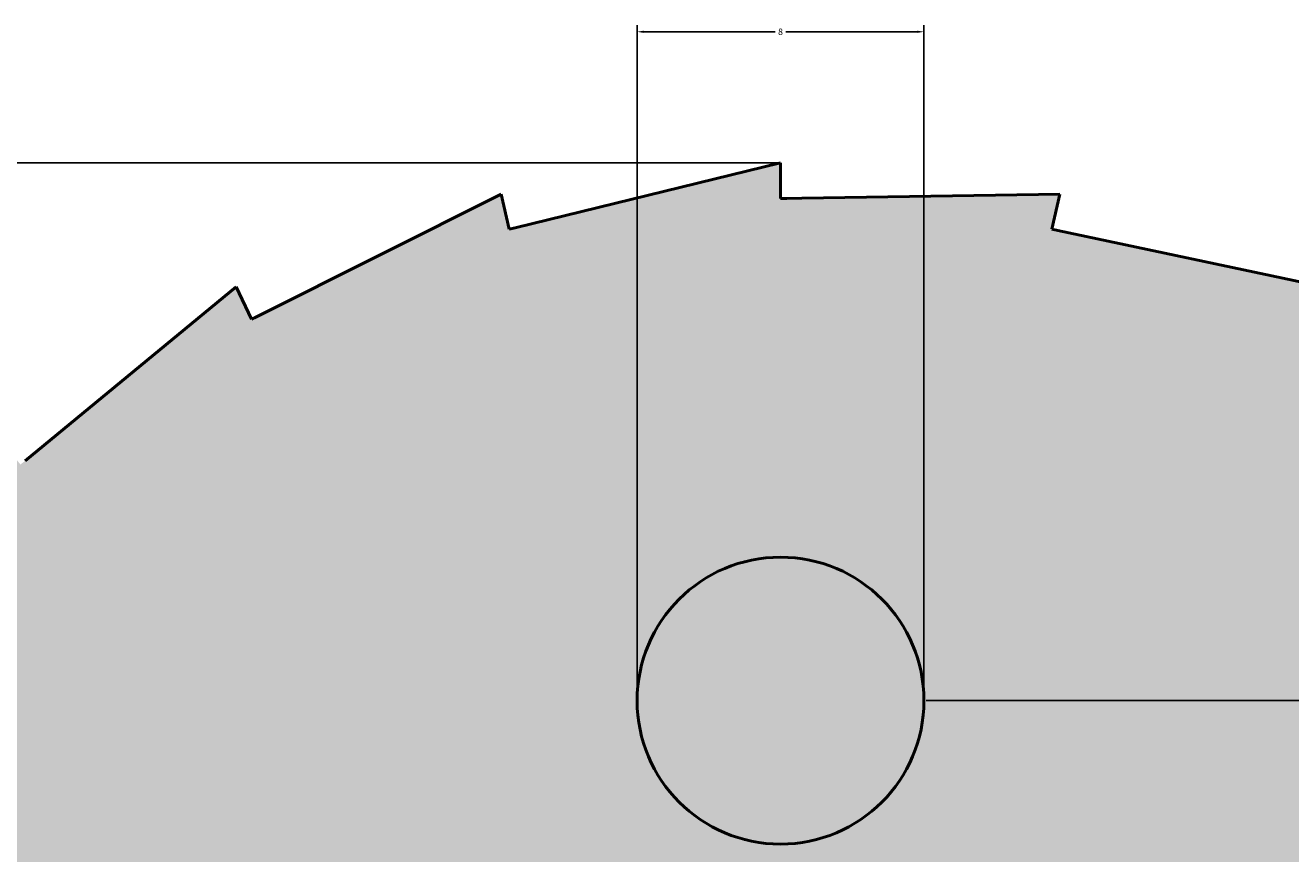
# Model space of a CAD drawing. Units: millimetres. Extents: x 2943.6 to 3032.7, y 1562 to 1639.7.
# Tile 6 of 9: x 2961.4 to 2996.7, y 1616.6 to 1639.7. Entities that reach past the tile are written whole.
import ezdxf

# ---------------------------------------------------------------- set-up
doc = ezdxf.new("R2010")
doc.units = ezdxf.units.MM
doc.layers.add('M-DIMS', color=2, linetype='Continuous', lineweight=18)
doc.layers.add('M-OUTL', color=7, linetype='Continuous', lineweight=50)
doc.layers.add('M-HATC', color=7, linetype='Continuous', lineweight=18, true_color=0xffffff)
doc.styles.get("Standard").update_dxf_attribs({"font": 'arial.ttf'})
doc.dimstyles.get("Standard").update_dxf_attribs({"dimtxt": 0.18, "dimasz": 0.18, "dimexe": 0.18, "dimexo": 0.0625, "dimgap": 0.09, "dimtad": 0, "dimtih": 1, "dimtoh": 1, "dimdec": 4, "dimzin": 0, "dimdsep": 46, "dimtxsty": 'Standard', "dimcen": 0.09, "dimadec": 0, "dimazin": 0, "dimtfac": 1, "dimtdec": 4, "dimtofl": 0, "dimtmove": 0, "dimatfit": 3, "dimfxl": 1, "dimtolj": 1, "dimtzin": 0, "dimarcsym": 0})

# ---------------------------------------------------------------- blocks, each defined once
blk = doc.blocks.new('*U1')
blk.add_circle((0, 0), 4)
blk = doc.blocks.new('*U2')
at = {"layer": 'M-OUTL', "color": 0, "linetype": 'ByBlock', "lineweight": -2, "transparency": 16777216}
blk.add_blockref('*U1', (2982.469, 1620.848), dxfattribs=at)
blk = doc.blocks.new('*D4')
at = {"layer": 'Defpoints', "color": 0, "transparency": 16777216}
for p in [(2943.819, 1635.848), (2982.469, 1635.848), (2982.469, 1565.848)]:
    blk.add_point(p, dxfattribs=at)
at = {"layer": 'M-DIMS', "color": 0, "lineweight": -2, "transparency": 16777216}
for p, q in [((2982.407, 1635.848), (2943.639, 1635.848)), ((2943.819, 1635.668), (2943.819, 1601.03)), ((2943.819, 1566.028), (2943.819, 1600.666)), ((2982.407, 1565.848), (2943.639, 1565.848))]:
    blk.add_line(p, q, dxfattribs=at)
at = {"layer": 'M-DIMS', "color": 0, "transparency": 16777216}
for points in [[(2943.789, 1635.668), (2943.849, 1635.668), (2943.819, 1635.848)], [(2943.789, 1566.028), (2943.849, 1566.028), (2943.819, 1565.848)]]:
    blk.add_solid(points, dxfattribs=at)
at = {"layer": 'M-DIMS', "color": 0, "transparency": 16777216, "insert": (2943.819, 1600.848), "char_height": 0.18, "attachment_point": 5}
blk.add_mtext('\\A1;70', dxfattribs=at)
blk = doc.blocks.new('*D5')
at = {"layer": 'Defpoints', "color": 0, "transparency": 16777216}
for p in [(2986.469, 1620.848), (3021.119, 1620.848), (2986.469, 1580.848)]:
    blk.add_point(p, dxfattribs=at)
at = {"layer": 'M-DIMS', "color": 0, "lineweight": -2, "transparency": 16777216}
for p, q in [((2986.532, 1620.848), (3021.299, 1620.848)), ((3021.119, 1620.668), (3021.119, 1601.03)), ((3021.119, 1581.028), (3021.119, 1600.666)), ((2986.532, 1580.848), (3021.299, 1580.848))]:
    blk.add_line(p, q, dxfattribs=at)
at = {"layer": 'M-DIMS', "color": 0, "transparency": 16777216}
for points in [[(3021.089, 1620.668), (3021.149, 1620.668), (3021.119, 1620.848)], [(3021.089, 1581.028), (3021.149, 1581.028), (3021.119, 1580.848)]]:
    blk.add_solid(points, dxfattribs=at)
at = {"layer": 'M-DIMS', "color": 0, "transparency": 16777216, "insert": (3021.119, 1600.848), "char_height": 0.18, "attachment_point": 5}
blk.add_mtext('\\A1;40', dxfattribs=at)
blk = doc.blocks.new('*D7')
at = {"layer": 'Defpoints', "color": 0, "transparency": 16777216}
for p in [(2986.469, 1639.498), (2978.469, 1620.848), (2986.469, 1620.848)]:
    blk.add_point(p, dxfattribs=at)
at = {"layer": 'M-DIMS', "color": 0, "lineweight": -2, "transparency": 16777216}
for p, q in [((2978.469, 1620.911), (2978.469, 1639.678)), ((2986.469, 1620.911), (2986.469, 1639.678)), ((2978.649, 1639.498), (2982.32, 1639.498)), ((2986.289, 1639.498), (2982.619, 1639.498))]:
    blk.add_line(p, q, dxfattribs=at)
at = {"layer": 'M-DIMS', "color": 0, "transparency": 16777216}
for points in [[(2978.649, 1639.528), (2978.649, 1639.468), (2978.469, 1639.498)], [(2986.289, 1639.528), (2986.289, 1639.468), (2986.469, 1639.498)]]:
    blk.add_solid(points, dxfattribs=at)
at = {"layer": 'M-DIMS', "color": 0, "transparency": 16777216, "insert": (2982.469, 1639.498), "char_height": 0.18, "attachment_point": 5}
blk.add_mtext('\\A1;8', dxfattribs=at)
blk = doc.blocks.new('*D10')
at = {"layer": 'Defpoints', "color": 0, "transparency": 16777216}
for p in [(3013.14, 1615.522), (2982.469, 1600.848)]:
    blk.add_point(p, dxfattribs=at)
at = {"layer": 'M-DIMS', "color": 0, "lineweight": -2, "transparency": 16777216}
for p, q in [((3031.542, 1624.326), (3013.302, 1615.6)), ((3031.722, 1624.326), (3031.542, 1624.326)), ((2982.379, 1600.848), (2982.559, 1600.848)), ((2982.469, 1600.758), (2982.469, 1600.938))]:
    blk.add_line(p, q, dxfattribs=at)
at = {"layer": 'M-DIMS', "color": 0, "transparency": 16777216}
blk.add_solid([(3013.289, 1615.627), (3013.315, 1615.573), (3013.14, 1615.522)], dxfattribs=at)
at = {"layer": 'M-DIMS', "color": 0, "transparency": 16777216, "insert": (3032.292, 1624.326), "char_height": 0.18, "attachment_point": 5}
blk.add_mtext('\\A1;28X R34', dxfattribs=at)

msp = doc.modelspace()

# ---------------------------------------------------------------- hatches: boundary and pattern name
at = {"layer": 'M-HATC'}
h = msp.add_hatch(color=256, dxfattribs=at)
h.set_gradient(color1=(0, 0, 255), color2=(255, 255, 0), tint=1, name='INVCURVED')
h.paths.add_polyline_path([(2949.361, 1608.583, 0.001279), (2949.322, 1608.414), (2948.347, 1608.637), (2948.473, 1600.848), (2947.469, 1600.848), (2949.283, 1593.452, 0.001279), (2949.322, 1593.283), (2948.347, 1593.06), (2951.761, 1586.253, 0.001279), (2951.836, 1586.096), (2950.935, 1585.662), (2955.779, 1579.786, 0.001279), (2955.887, 1579.65), (2955.105, 1579.026), (2961.135, 1574.375, 0.001279), (2961.271, 1574.266), (2960.647, 1573.484), (2967.561, 1570.291, 0.001279), (2967.717, 1570.215), (2967.283, 1569.314), (2974.734, 1567.74, 0.001279), (2974.904, 1567.701), (2974.681, 1566.726), (2982.295, 1566.849, 0.001279), (2982.469, 1566.848), (2982.469, 1565.848), (2989.865, 1567.662, 0.001279), (2990.035, 1567.701), (2990.258, 1566.726), (2997.064, 1570.14, 0.001279), (2997.221, 1570.215), (2997.655, 1569.314), (3003.532, 1574.158, 0.001279), (3003.668, 1574.266), (3004.291, 1573.484), (3008.943, 1579.514, 0.001279), (3009.052, 1579.65), (3009.833, 1579.026), (3013.026, 1585.94, 0.001279), (3013.102, 1586.096), (3014.003, 1585.662), (3015.578, 1593.113, 0.001279), (3015.617, 1593.283), (3016.592, 1593.06), (3016.469, 1600.674, 0.001279), (3016.469, 1600.848), (3017.469, 1600.848), (3015.655, 1608.244, 0.001279), (3015.617, 1608.414), (3016.592, 1608.637), (3013.177, 1615.443, 0.001279), (3013.102, 1615.6), (3014.003, 1616.034), (3009.16, 1621.911, 0.001279), (3009.052, 1622.047), (3009.833, 1622.67), (3003.804, 1627.322, 0.001279), (3003.668, 1627.431), (3004.291, 1628.212), (2997.378, 1631.405, 0.001279), (2997.221, 1631.481), (2997.655, 1632.382), (2990.204, 1633.957, 0.001279), (2990.035, 1633.996), (2990.258, 1634.971), (2982.469, 1634.845), (2982.469, 1635.848), (2975.073, 1634.034, 0.001279), (2974.904, 1633.996), (2974.681, 1634.971), (2967.874, 1631.556, 0.001279), (2967.717, 1631.481), (2967.283, 1632.382), (2961.407, 1627.539, 0.001279), (2961.271, 1627.431), (2960.647, 1628.212), (2955.996, 1622.183, 0.001279), (2955.887, 1622.047), (2955.105, 1622.67), (2951.912, 1615.757, 0.001279), (2951.836, 1615.6), (2950.935, 1616.034)])
h.paths.add_polyline_path([(2969.149, 1610.848, -1), (2961.149, 1610.848, -1)], flags=16)
h.paths.add_polyline_path([(2969.149, 1590.848, -1), (2961.149, 1590.848, -1)], flags=16)
h.paths.add_polyline_path([(2992.469, 1600.848, -1), (2972.469, 1600.848, -1)], flags=16)
h.paths.add_polyline_path([(2978.469, 1620.848, -1), (2986.469, 1620.848, -1)], flags=16)
h.paths.add_polyline_path([(2981.469, 1605.236), (2981.469, 1606.848), (2983.469, 1606.848), (2983.469, 1605.236, -8.887482)], flags=0)
h.paths.add_polyline_path([(2986.469, 1580.848, -1), (2978.469, 1580.848, -1)], flags=16)
h.paths.add_polyline_path([(3003.79, 1610.848, -1), (2995.79, 1610.848, -1)], flags=16)
h.paths.add_polyline_path([(3003.79, 1590.848, -1), (2995.79, 1590.848, -1)], flags=16)
h = msp.add_hatch(color=256, dxfattribs=at)
h.paths.add_polyline_path([(2978.469, 1620.848, 1), (2986.469, 1620.848, 1)])
h.paths.add_polyline_path([(2995.79, 1610.848, 1), (3003.79, 1610.848, 1)])
h.paths.add_polyline_path([(3003.79, 1590.848, 1), (2995.79, 1590.848, 1)])
h.paths.add_polyline_path([(2986.469, 1580.848, 1), (2978.469, 1580.848, 1)])
h.paths.add_polyline_path([(2969.149, 1590.848, 1), (2961.149, 1590.848, 1)])
h.paths.add_polyline_path([(2961.149, 1610.848, 1), (2969.149, 1610.848, 1)])

# ---------------------------------------------------------------- linework, layer by layer
at = {"layer": 'M-OUTL'}
for p, q in [((2975.073, 1634.034), (2982.469, 1635.848)), ((2982.469, 1635.848), (2982.469, 1634.845)), ((2982.469, 1634.848), (2982.469, 1635.848)), ((2967.874, 1631.556), (2974.681, 1634.971)), ((2974.904, 1633.996), (2974.681, 1634.971)), ((2982.469, 1634.845), (2990.258, 1634.971)), ((2990.035, 1633.996), (2990.258, 1634.971)), ((2990.204, 1633.957), (2997.655, 1632.382)), ((2961.407, 1627.539), (2967.283, 1632.382)), ((2967.717, 1631.481), (2967.283, 1632.382))]:
    msp.add_line(p, q, dxfattribs=at)
for start, end in [(89.7069, 90), (102.564, 102.8571), (76.8498, 77.1429), (115.4212, 115.7143)]:
    msp.add_arc((2982.469, 1600.848), 34, start, end, dxfattribs=at)

# ---------------------------------------------------------------- block references
msp.add_blockref('*U2', (0, 0), dxfattribs=at)

# ---------------------------------------------------------------- dimensions: what is measured, and where the dimension line sits
at = {"layer": 'M-DIMS'}
dim = msp.add_linear_dim(base=(2986.469, 1639.498), p1=(2978.469, 1620.848), p2=(2986.469, 1620.848), dimstyle='Standard', override={"dimdec": 0, "dimlfac": 1, "dimrnd": 0, "dimzin": 0, "dimdsep": 46, "dimlunit": 2}, dxfattribs=at)
dim.commit()
dim.dimension.update_dxf_attribs({"geometry": '*D7', "text_midpoint": (2982.469, 1639.498)})
for base, p1, p2, picture, middle in [((2943.819, 1635.848), (2982.469, 1565.848), (2982.469, 1635.848), '*D4', (2943.819, 1600.848)), ((3021.119, 1620.848), (2986.469, 1580.848), (2986.469, 1620.848), '*D5', (3021.119, 1600.848))]:
    dim = msp.add_linear_dim(base=base, p1=p1, p2=p2, angle=90, dimstyle='Standard', override={"dimdec": 0, "dimlfac": 1, "dimrnd": 0, "dimzin": 0, "dimdsep": 46, "dimlunit": 2}, dxfattribs=at)
    dim.commit()
    dim.dimension.update_dxf_attribs({"geometry": picture, "text_midpoint": middle})
dim = msp.add_radius_dim(center=(2982.469, 1600.848), mpoint=(3013.14, 1615.522), text='28X <>', dimstyle='Standard', override={"dimdec": 0, "dimlfac": 1, "dimrnd": 0, "dimzin": 0, "dimdsep": 46, "dimlunit": 2}, dxfattribs=at)
dim.commit()
dim.dimension.update_dxf_attribs({"geometry": '*D10', "text_midpoint": (3032.292, 1624.326), "dimtype": 164})

doc.saveas('drawing.dxf')
